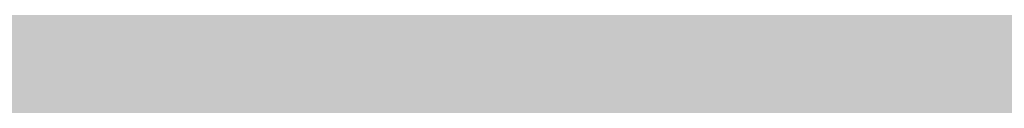
# Model space of a CAD drawing. Units: feet. Extents: x 3168 to 4724, y 827 to 1477.
# Tile 66 of 256: x 3273.15625 to 3273.17306, y 1099.01485 to 1099.01628. Entities that reach past the tile are written whole.
import ezdxf

# ---------------------------------------------------------------- set-up
doc = ezdxf.new("R2010")
doc.units = ezdxf.units.FT
doc.layers.add('A-ELEV', color=7, linetype='Continuous', lineweight=35)
doc.layers.add('A-ELEV-PATT', color=8, linetype='Continuous', lineweight=13)

msp = doc.modelspace()

# ---------------------------------------------------------------- hatches: boundary and pattern name
at = {"layer": 'A-ELEV-PATT'}
h = msp.add_hatch(color=256, dxfattribs=at)
h.dxf.hatch_style = 1
edge = h.paths.add_edge_path()
edge.add_ellipse((3552.905762, 979.220141), major_axis=(36.744924, 0), ratio=0.484848485, start_angle=0, end_angle=360)
edge = h.paths.add_edge_path()
edge.add_ellipse((3559.891637, 929.252282), major_axis=(36.744924, 0), ratio=0.484848485, start_angle=0, end_angle=360)
edge = h.paths.add_edge_path()
edge.add_line((3299.31681, 1198.606081), (3479.916714, 1198.606081))
edge.add_line((3479.916714, 1198.606081), (3479.916714, 1209.86857))
edge.add_spline(control_points=[(3479.916714, 1209.86857), (3464.301157, 1209.86857), (3448.685601, 1209.86857), (3410.949139, 1209.86857), (3388.828234, 1209.86857), (3355.646876, 1209.86857), (3344.586423, 1209.86857), (3327.995745, 1209.86857), (3322.465518, 1209.86857), (3314.170179, 1209.86857), (3311.405066, 1209.86857), (3307.257396, 1209.86857), (3305.874839, 1209.86857), (3303.801005, 1209.86857), (3303.109726, 1209.86857), (3302.072809, 1209.86857), (3301.72717, 1209.86857), (3301.208711, 1209.86857), (3301.035891, 1209.86857), (3300.776662, 1209.86857), (3300.690252, 1209.86857), (3300.560638, 1209.86857), (3300.517433, 1209.86857), (3300.452625, 1209.86857), (3300.431023, 1209.86857), (3300.398619, 1209.86857), (3300.387818, 1209.86857), (3300.366216, 1209.86857), (3300.345676, 1209.86857), (3300.345548, 1209.86857), (3300.345505, 1209.86857), (3300.343304, 1209.86857), (3300.341146, 1209.868571), (3300.337909, 1209.868571), (3300.33683, 1209.868572), (3300.333942, 1209.868573), (3300.332133, 1209.868574), (3300.325515, 1209.868577), (3300.320706, 1209.868581), (3300.310925, 1209.868592), (3300.305952, 1209.868598), (3300.290511, 1209.868623), (3300.280045, 1209.868646), (3300.232425, 1209.868777), (3300.195298, 1209.868954), (3299.951068, 1209.870608), (3299.744824, 1209.874326), (3299.436827, 1209.883257), (3299.334389, 1209.886792), (3299.181079, 1209.89292), (3299.130033, 1209.895099), (3298.652217, 1209.916801), (3298.22946, 1209.945718), (3297.601631, 1210.002367), (3297.393404, 1210.023464), (3297.082652, 1210.058309), (3296.979332, 1210.070458), (3296.292954, 1210.154861), (3295.718148, 1210.243356), (3294.868717, 1210.39885), (3294.5877, 1210.454478), (3294.169341, 1210.543349), (3294.030415, 1210.573878), (3291.707149, 1211.1012), (3289.65359, 1211.813435), (3285.776259, 1213.563988), (3283.95141, 1214.603478), (3280.512159, 1216.98008), (3278.897241, 1218.317592), (3276.379914, 1220.829489), (3275.416042, 1221.917738), (3274.039342, 1223.7077), (3273.581043, 1224.349535), (3273.143228, 1225.016316)], knot_values=[39.119033, 39.119033, 39.119033, 39.119033, 39.286353, 39.286353, 39.523379, 39.523379, 39.641892, 39.641892, 39.701148, 39.701148, 39.730777, 39.730777, 39.745591, 39.745591, 39.752998, 39.752998, 39.756701, 39.756701, 39.758553, 39.758553, 39.759479, 39.759479, 39.759942, 39.759942, 39.760173, 39.760173, 39.760289, 39.760289, 39.760405, 39.760405, 39.760463, 39.760463, 39.763389, 39.763389, 39.764851, 39.764851, 39.767304, 39.767304, 39.773825, 39.773825, 39.78057, 39.78057, 39.79477, 39.79477, 39.845194, 39.845194, 40.126715, 40.126715, 40.267476, 40.267476, 40.337856, 40.337856, 40.927023, 40.927023, 41.221606, 41.221606, 41.368898, 41.368898, 42.202622, 42.202622, 42.619485, 42.619485, 42.827916, 42.827916, 46.118323, 46.118323, 49.408731, 49.408731, 52.699139, 52.699139, 54.927489, 54.927489, 56.104228, 56.104228, 56.104228, 56.104228], weights=[1, 1, 1, 1, 1, 1, 1, 1, 1, 1, 1, 1, 1, 1, 1, 1, 1, 1, 1, 1, 1, 1, 1, 1, 1, 1, 1, 1, 1, 1, 1, 1, 1, 1, 1, 1, 1, 1, 1, 1, 1, 1, 1, 1, 1, 1, 1, 1, 1, 1, 1, 1, 1, 1, 1, 1, 1, 1, 1, 1, 1, 1, 1, 1, 1, 1, 1, 1, 1, 1, 1, 1, 1, 1], degree=3, periodic=0)
edge.add_line((3273.143228, 1225.016316), (3273.143228, 1099.016316))
edge.add_line((3273.143228, 1099.016316), (3299.31681, 1099.016316))
edge.add_line((3299.31681, 1099.016316), (3299.31681, 1198.606081))
edge = h.paths.add_edge_path()
edge.add_line((3304.758443, 1324.15806), (3479.916714, 1324.15806))
edge.add_line((3479.916714, 1324.15806), (3479.916714, 1335.714618))
edge.add_line((3479.916714, 1335.714618), (3269.161628, 1335.714618))
edge.add_spline(control_points=[(3269.161628, 1335.714618), (3264.024231, 1335.714618), (3258.364118, 1328.958189), (3259.264311, 1323.900274)], knot_values=[0, 0, 0, 0, 15.412191, 15.412191, 15.412191, 15.412191], degree=3, periodic=0)
edge.add_line((3259.264311, 1323.900274), (3265.516849, 1288.769135))
edge.add_line((3265.516849, 1288.769135), (3275.265103, 1261.545626))
edge.add_line((3275.265103, 1261.545626), (3304.758443, 1261.545626))
edge.add_line((3304.758443, 1261.545626), (3304.758443, 1324.15806))
h = msp.add_hatch(color=256, dxfattribs=at)
h.dxf.hatch_style = 1
h.paths.add_polyline_path([(3384.525247, 1099.016316), (3335.029168, 1099.016316), (3299.31681, 1099.016316), (3273.143228, 1099.016316), (3217.565364, 1099.016316), (3168.069285, 827.11626), (3335.029168, 827.11626)])

# ---------------------------------------------------------------- linework, layer by layer
at = {"layer": 'A-ELEV'}
msp.add_open_spline([(3808.5202, 1099.016316), (3808.5202, 1141.413235), (3808.5202, 1183.810154), (3808.5202, 1226.635324), (3808.5202, 1227.063576), (3808.5202, 1227.491828), (3811.491871, 1248.994673), (3814.463542, 1270.497518), (3817.46523, 1292.217564), (3817.495247, 1292.434764), (3817.525264, 1292.651964), (3817.572801, 1310.106748), (3817.620339, 1327.561532), (3817.667877, 1345.016316), (3817.667877, 1345.457962), (3817.667877, 1345.899608), (3817.667877, 1346.456047), (3817.667877, 1346.57084), (3817.667877, 1346.752887), (3817.667877, 1346.820142), (3817.667877, 1346.93487), (3817.667877, 1346.982345), (3817.667877, 1347.038587), (3817.667877, 1347.047356), (3817.667877, 1347.073661), (3817.667877, 1347.059303), (3817.667877, 1347.061545), (3817.667876, 1347.062667), (3817.667875, 1347.066031), (3817.667874, 1347.068274), (3817.66787, 1347.075001), (3817.667866, 1347.079486), (3817.667849, 1347.092937), (3817.667833, 1347.101902), (3817.667766, 1347.12879), (3817.667699, 1347.146705), (3817.667432, 1347.200421), (3817.667165, 1347.236192), (3817.6661, 1347.343385), (3817.665038, 1347.414686), (3817.660812, 1347.628095), (3817.656608, 1347.769708), (3817.63997, 1348.192487), (3817.623509, 1348.471586), (3817.559094, 1349.300067), (3817.496121, 1349.840588), (3817.255432, 1351.424156), (3817.026318, 1352.428785), (3816.306871, 1354.888914), (3815.743745, 1356.268727), (3814.463959, 1358.81921), (3813.746413, 1359.990968), (3812.195838, 1362.172343), (3811.362245, 1363.182124), (3809.588836, 1365.069009), (3808.648816, 1365.946105), (3806.654262, 1367.579616), (3805.599702, 1368.336154), (3803.352891, 1369.722327), (3802.160535, 1370.352386), (3799.600813, 1371.453586), (3798.232688, 1371.925481), (3795.280084, 1372.634624), (3793.693148, 1372.872068), (3791.869441, 1372.92648), (3791.740861, 1372.92922), (3791.353371, 1372.934101), (3791.092707, 1372.932901), (3790.304116, 1372.915068), (3789.769543, 1372.884195), (3789.20919, 1372.830236), (3789.190622, 1372.828424), (3789.134892, 1372.822912), (3789.097705, 1372.819137), (3789.048445, 1372.814008), (3789.0364, 1372.812743), (3789.000256, 1372.808918), (3788.976147, 1372.806325), (3788.949405, 1372.803404), (3788.946786, 1372.803118), (3788.942567, 1372.802655), (3788.940967, 1372.80248), (3788.938572, 1372.802217), (3788.937777, 1372.802129), (3788.935391, 1372.801867), (3788.867535, 1372.794402), (3788.756866, 1372.782228), (3788.701532, 1372.776141), (3788.53553, 1372.75788), (3788.424861, 1372.745707), (3788.092856, 1372.709185), (3787.871519, 1372.684837), (3787.207509, 1372.611793), (3786.764835, 1372.563097), (3785.436814, 1372.417009), (3784.551467, 1372.319617), (3781.895425, 1372.027442), (3780.12473, 1371.832658), (3774.812646, 1371.248307), (3771.271256, 1370.858739), (3760.647088, 1369.690037), (3753.56431, 1368.910902), (3732.315973, 1366.573498), (3718.150416, 1365.015228), (3694.006758, 1362.359326), (3684.028657, 1361.261694), (3674.050557, 1360.164062), (3664.600662, 1360.164062), (3655.150767, 1360.164062), (3626.801081, 1360.164062), (3607.901291, 1360.164062), (3551.20192, 1360.164062), (3513.40234, 1360.164062), (3467.725182, 1360.164062), (3459.847604, 1360.164062), (3436.214873, 1360.164062), (3420.459718, 1360.164062), (3373.194255, 1360.164062), (3341.683946, 1360.164062), (3302.848162, 1360.164062), (3295.522686, 1360.164062), (3286.038292, 1360.164062), (3283.879372, 1360.164062), (3277.402613, 1360.164062), (3273.084773, 1360.164062), (3267.732851, 1360.164062), (3266.698768, 1360.164062), (3263.59652, 1360.164062), (3261.528355, 1360.164062), (3259.236943, 1360.164062), (3259.013697, 1360.164062), (3258.343958, 1360.164062), (3257.897466, 1360.164062), (3257.430998, 1360.164062), (3257.411022, 1360.164062), (3257.370573, 1360.164062), (3257.37547, 1360.164062), (3257.374598, 1360.164062), (3257.373937, 1360.164062), (3257.371956, 1360.164062), (3257.370635, 1360.164061), (3257.366673, 1360.16406), (3257.364032, 1360.164059), (3257.356109, 1360.164053), (3257.350828, 1360.164047), (3257.334987, 1360.164023), (3257.32443, 1360.163998), (3257.292769, 1360.163899), (3257.271676, 1360.163799), (3257.208439, 1360.163398), (3257.166337, 1360.162995), (3257.040206, 1360.161388), (3256.956349, 1360.159783), (3256.705504, 1360.153393), (3256.53924, 1360.147036), (3256.04357, 1360.121916), (3255.717296, 1360.097102), (3254.752446, 1360.000481), (3254.127968, 1359.906513), (3252.180067, 1359.525332), (3250.941574, 1359.143991), (3248.670175, 1358.24329), (3247.635739, 1357.723834), (3245.732632, 1356.603471), (3244.863388, 1356.00206), (3243.253108, 1354.742865), (3242.511972, 1354.084731), (3240.751052, 1352.344781), (3239.800961, 1351.229574), (3238.087769, 1348.87244), (3237.324685, 1347.630355), (3235.98251, 1344.971632), (3235.402205, 1343.554907), (3234.591081, 1340.815458), (3234.310882, 1339.54355), (3233.97649, 1336.802561), (3233.922113, 1335.330877), (3234.148916, 1332.591269), (3234.349529, 1331.367201), (3234.719893, 1329.999367), (3234.752423, 1329.883362), (3234.853619, 1329.534797), (3234.925892, 1329.301685), (3235.024836, 1329.002552), (3235.046924, 1328.936928), (3235.077639, 1328.847239), (3235.085924, 1328.823198), (3235.110939, 1328.751064), (3235.127828, 1328.702962), (3235.147992, 1328.646242), (3235.151059, 1328.637632), (3235.156096, 1328.623526), (3235.158061, 1328.61803), (3235.160209, 1328.61203), (3235.165612, 1328.596943), (3235.180099, 1328.556486), (3235.190263, 1328.528101), (3235.220756, 1328.442946), (3235.241084, 1328.386176), (3235.302069, 1328.215865), (3235.342726, 1328.102325), (3235.464696, 1327.761704), (3235.54601, 1327.534623), (3235.78995, 1326.853381), (3235.952577, 1326.39922), (3236.440459, 1325.036736), (3236.765713, 1324.128414), (3237.741475, 1321.403446), (3238.391983, 1319.586801), (3240.343508, 1314.136866), (3241.644525, 1310.503576), (3245.547574, 1299.603706), (3248.149607, 1292.337126), (3255.955706, 1270.537385), (3261.159772, 1256.004225), (3267.387618, 1238.612001), (3268.411397, 1235.752937), (3269.510378, 1232.683864), (3269.585579, 1232.473854), (3269.706612, 1232.135851), (3269.752444, 1232.007857), (3269.827329, 1231.79873), (3269.856382, 1231.717595), (3269.906325, 1231.578122), (3269.927215, 1231.519782), (3269.972468, 1231.393406), (3269.996831, 1231.325368), (3270.026503, 1231.242506), (3270.031811, 1231.227681), (3270.040282, 1231.204024), (3270.039224, 1231.206979), (3270.039359, 1231.206601), (3270.039427, 1231.206412), (3270.03963, 1231.205846), (3270.039765, 1231.205468), (3270.040171, 1231.204335), (3270.040442, 1231.203579), (3270.041254, 1231.201313), (3270.041796, 1231.199802), (3270.04342, 1231.195269), (3270.044504, 1231.192248), (3270.047756, 1231.183185), (3270.049926, 1231.177145), (3270.056442, 1231.159028), (3270.060793, 1231.146957), (3270.073867, 1231.110761), (3270.082613, 1231.086656), (3270.108936, 1231.014413), (3270.1266, 1230.96635), (3270.179934, 1230.822457), (3270.215947, 1230.726923), (3270.325323, 1230.441508), (3270.400026, 1230.252811), (3270.629249, 1229.691444), (3270.788883, 1229.323501), (3271.286488, 1228.238319), (3271.6431, 1227.539755), (3272.775859, 1225.515277), (3273.614169, 1224.260502), (3275.416042, 1221.917738), (3276.379914, 1220.829489), (3278.897241, 1218.317592), (3280.512159, 1216.98008), (3283.95141, 1214.603478), (3285.776259, 1213.563988), (3289.65359, 1211.813435), (3291.707149, 1211.1012), (3294.030415, 1210.573878), (3294.169341, 1210.543349), (3294.5877, 1210.454478), (3294.868717, 1210.39885), (3295.718148, 1210.243356), (3296.292954, 1210.154861), (3296.979332, 1210.070458), (3297.082652, 1210.058309), (3297.393404, 1210.023464), (3297.601631, 1210.002367), (3298.22946, 1209.945718), (3298.652217, 1209.916801), (3299.130033, 1209.895099), (3299.181079, 1209.89292), (3299.334389, 1209.886792), (3299.436827, 1209.883257), (3299.744824, 1209.874326), (3299.951068, 1209.870608), (3300.195298, 1209.868954), (3300.232425, 1209.868777), (3300.280045, 1209.868646), (3300.290511, 1209.868623), (3300.305952, 1209.868598), (3300.310925, 1209.868592), (3300.320706, 1209.868581), (3300.325515, 1209.868577), (3300.332133, 1209.868574), (3300.333942, 1209.868573), (3300.33683, 1209.868572), (3300.337909, 1209.868571), (3300.341146, 1209.868571), (3300.343304, 1209.86857), (3300.345505, 1209.86857), (3300.345548, 1209.86857), (3300.345676, 1209.86857), (3300.366216, 1209.86857), (3300.387818, 1209.86857), (3300.398619, 1209.86857), (3300.431023, 1209.86857), (3300.452625, 1209.86857), (3300.517433, 1209.86857), (3300.560638, 1209.86857), (3300.690252, 1209.86857), (3300.776662, 1209.86857), (3301.035891, 1209.86857), (3301.208711, 1209.86857), (3301.72717, 1209.86857), (3302.072809, 1209.86857), (3303.109726, 1209.86857), (3303.801005, 1209.86857), (3305.874839, 1209.86857), (3307.257396, 1209.86857), (3311.405066, 1209.86857), (3314.170179, 1209.86857), (3322.465518, 1209.86857), (3327.995745, 1209.86857), (3344.586423, 1209.86857), (3355.646876, 1209.86857), (3388.828234, 1209.86857), (3410.949139, 1209.86857), (3477.311855, 1209.86857), (3521.553665, 1209.86857), (3566.836184, 1209.86857), (3567.876892, 1209.86857), (3570.999017, 1209.86857), (3573.080433, 1209.86857), (3575.781396, 1209.86857), (3576.400943, 1209.86857), (3577.295821, 1209.86857), (3577.571152, 1209.86857), (3578.397146, 1209.86857), (3578.947808, 1209.86857), (3579.756491, 1209.86857), (3580.014511, 1209.86857), (3580.342737, 1209.86857), (3580.326865, 1209.86857), (3580.32717, 1209.86857), (3580.327323, 1209.86857), (3580.327781, 1209.86857), (3580.328086, 1209.86857), (3580.329002, 1209.86857), (3580.329613, 1209.86857), (3580.331445, 1209.86857), (3580.332667, 1209.86857), (3580.336332, 1209.868569), (3580.338775, 1209.868567), (3580.346107, 1209.868563), (3580.350995, 1209.868558), (3580.365663, 1209.86854), (3580.375445, 1209.868522), (3580.404801, 1209.868449), (3580.424386, 1209.868376), (3580.483183, 1209.868085), (3580.522437, 1209.867793), (3580.640361, 1209.866624), (3580.719195, 1209.865454), (3580.956315, 1209.860766), (3581.115222, 1209.85607), (3581.594164, 1209.83723), (3581.916419, 1209.818331), (3582.889947, 1209.742428), (3583.547986, 1209.666169), (3585.531827, 1209.360617), (3586.867216, 1209.053886), (3589.471545, 1208.252472), (3590.740241, 1207.757852), (3591.995451, 1207.158802), (3592.057809, 1207.12874), (3592.244242, 1207.037954), (3592.367676, 1206.976632), (3592.73528, 1206.790359), (3592.976752, 1206.663101), (3593.244539, 1206.516441), (3593.274731, 1206.499825), (3593.365115, 1206.449839), (3593.425113, 1206.416333), (3593.604314, 1206.315285), (3593.722725, 1206.247211), (3593.857212, 1206.168398), (3593.874362, 1206.158319), (3593.925741, 1206.128041), (3593.959899, 1206.107798), (3594.062086, 1206.046899), (3594.129827, 1206.006074), (3594.208436, 1205.958171), (3594.219683, 1205.951304), (3594.253391, 1205.930686), (3594.275819, 1205.916917), (3594.342972, 1205.875536), (3594.387563, 1205.847853), (3594.433616, 1205.81905), (3594.435256, 1205.818024), (3594.440175, 1205.814946), (3594.443453, 1205.812894), (3594.447123, 1205.810594), (3594.447516, 1205.810348), (3594.448695, 1205.80961), (3594.449481, 1205.809117), (3594.450366, 1205.808562), (3594.450466, 1205.8085), (3594.4506, 1205.808415), (3594.467399, 1205.797887), (3594.493269, 1205.781674), (3594.506204, 1205.773568), (3594.545008, 1205.749248), (3594.570878, 1205.733035), (3594.648487, 1205.684396), (3594.700226, 1205.651969), (3594.855444, 1205.554691), (3594.958922, 1205.489839), (3595.269357, 1205.295282), (3595.476314, 1205.165577), (3596.097185, 1204.776463), (3596.511099, 1204.517054), (3597.752841, 1203.738826), (3598.580669, 1203.220007), (3601.064152, 1201.663551), (3602.719807, 1200.625914), (3607.686774, 1197.513002), (3610.998085, 1195.437727), (3620.932018, 1189.211903), (3627.55464, 1185.061354), (3647.422507, 1172.609707), (3660.667751, 1164.308608), (3700.403484, 1139.405313), (3726.893973, 1122.803116), (3757.205715, 1103.806052), (3761.02697, 1101.411184), (3764.848224, 1099.016316), (3745.328271, 1099.016316), (3725.808319, 1099.016316), (3706.288366, 1099.016316), (3706.288366, 1108.453237), (3706.288366, 1117.890158), (3706.288366, 1127.327079), (3710.750754, 1127.327079), (3715.213143, 1127.327079), (3719.675531, 1127.327079)], degree=3, knots=[0, 0, 0, 0, 0.982037, 0.982037, 0.991957, 0.991957, 0.991957, 1.966522, 1.966522, 1.976367, 1.976367, 1.976367, 2.976367, 2.976367, 2.976367, 3.00169, 3.00169, 3.008272, 3.008272, 3.012129, 3.012129, 3.014851, 3.014851, 3.015353, 3.015353, 3.016359, 3.016359, 3.017365, 3.017365, 3.019376, 3.019376, 3.023398, 3.023398, 3.031442, 3.031442, 3.047531, 3.047531, 3.079708, 3.079708, 3.144063, 3.144063, 3.272772, 3.272772, 3.53019, 3.53019, 4.045026, 4.045026, 5.074698, 5.074698, 6.700878, 6.700878, 8.327058, 8.327058, 9.953238, 9.953238, 11.579418, 11.579418, 13.205598, 13.205598, 14.831778, 14.831778, 16.457958, 16.457958, 18.084138, 18.084138, 18.206872, 18.206872, 18.45234, 18.45234, 18.943275, 18.943275, 18.960093, 18.960093, 18.993729, 18.993729, 19.00461, 19.00461, 19.026374, 19.026374, 19.028737, 19.028737, 19.03018, 19.03018, 19.030897, 19.030897, 19.032332, 19.032332, 19.033766, 19.033766, 19.036636, 19.036636, 19.042374, 19.042374, 19.053851, 19.053851, 19.076805, 19.076805, 19.122714, 19.122714, 19.21453, 19.21453, 19.398163, 19.398163, 19.765429, 19.765429, 20.024128, 20.024128, 20.024128, 20.092031, 20.092031, 20.227836, 20.227836, 20.499446, 20.499446, 20.556051, 20.556051, 20.66926, 20.66926, 20.895678, 20.895678, 20.948316, 20.948316, 20.963829, 20.963829, 20.994855, 20.994855, 21.002285, 21.002285, 21.017146, 21.017146, 21.01875, 21.01875, 21.021959, 21.021959, 21.022102, 21.022102, 21.022249, 21.022249, 21.022708, 21.022708, 21.023627, 21.023627, 21.025464, 21.025464, 21.029138, 21.029138, 21.036486, 21.036486, 21.051183, 21.051183, 21.080575, 21.080575, 21.139361, 21.139361, 21.256932, 21.256932, 21.492073, 21.492073, 21.962356, 21.962356, 23.01002, 23.01002, 24.057684, 24.057684, 25.105348, 25.105348, 26.153011, 26.153011, 27.776787, 27.776787, 29.400562, 29.400562, 31.024337, 31.024337, 32.278801, 32.278801, 33.533265, 33.533265, 34.467568, 34.467568, 34.553971, 34.553971, 34.726776, 34.726776, 34.775309, 34.775309, 34.793079, 34.793079, 34.82862, 34.82862, 34.834979, 34.834979, 34.839039, 34.839039, 34.839411, 34.839411, 34.840285, 34.840285, 34.842034, 34.842034, 34.845531, 34.845531, 34.852525, 34.852525, 34.866512, 34.866512, 34.894488, 34.894488, 34.950439, 34.950439, 35.062342, 35.062342, 35.286147, 35.286147, 35.733758, 35.733758, 35.821815, 35.821815, 35.828283, 35.828283, 35.832225, 35.832225, 35.834724, 35.834724, 35.836521, 35.836521, 35.838617, 35.838617, 35.839073, 35.839073, 35.839345, 35.839345, 35.839617, 35.839617, 35.840161, 35.840161, 35.841249, 35.841249, 35.843425, 35.843425, 35.847778, 35.847778, 35.856482, 35.856482, 35.873891, 35.873891, 35.908709, 35.908709, 35.978345, 35.978345, 36.117617, 36.117617, 36.396161, 36.396161, 36.953248, 36.953248, 38.067423, 38.067423, 40.295772, 40.295772, 42.524122, 42.524122, 45.81453, 45.81453, 49.104937, 49.104937, 52.395345, 52.395345, 52.603776, 52.603776, 53.020639, 53.020639, 53.854363, 53.854363, 54.001655, 54.001655, 54.296238, 54.296238, 54.885405, 54.885405, 54.955785, 54.955785, 55.096546, 55.096546, 55.378067, 55.378067, 55.42849, 55.42849, 55.442691, 55.442691, 55.449436, 55.449436, 55.455957, 55.455957, 55.458409, 55.458409, 55.459872, 55.459872, 55.462798, 55.462798, 55.462856, 55.462856, 55.462972, 55.462972, 55.463088, 55.463088, 55.463319, 55.463319, 55.463782, 55.463782, 55.464708, 55.464708, 55.46656, 55.46656, 55.470263, 55.470263, 55.47767, 55.47767, 55.492484, 55.492484, 55.522112, 55.522112, 55.581369, 55.581369, 55.699882, 55.699882, 55.936907, 55.936907, 56.410959, 56.410959, 56.42211, 56.42211, 56.444413, 56.444413, 56.451051, 56.451051, 56.454001, 56.454001, 56.459901, 56.459901, 56.462666, 56.462666, 56.463418, 56.463418, 56.464171, 56.464171, 56.465675, 56.465675, 56.468684, 56.468684, 56.474702, 56.474702, 56.486738, 56.486738, 56.51081, 56.51081, 56.558955, 56.558955, 56.655243, 56.655243, 56.847821, 56.847821, 57.232975, 57.232975, 58.003284, 58.003284, 59.543901, 59.543901, 62.625137, 62.625137, 68.787607, 68.787607, 74.950078, 74.950078, 75.27336, 75.27336, 75.919923, 75.919923, 77.213051, 77.213051, 77.377769, 77.377769, 77.707206, 77.707206, 78.366079, 78.366079, 78.462532, 78.462532, 78.655436, 78.655436, 79.041245, 79.041245, 79.105735, 79.105735, 79.234714, 79.234714, 79.492672, 79.492672, 79.502197, 79.502197, 79.521249, 79.521249, 79.523534, 79.523534, 79.528103, 79.528103, 79.528682, 79.528682, 79.528885, 79.528885, 79.529089, 79.529089, 79.529495, 79.529495, 79.530308, 79.530308, 79.531935, 79.531935, 79.535187, 79.535187, 79.541693, 79.541693, 79.554704, 79.554704, 79.580725, 79.580725, 79.632769, 79.632769, 79.736856, 79.736856, 79.94503, 79.94503, 80.361377, 80.361377, 80.421435, 80.421435, 80.421435, 81.421435, 81.421435, 81.421435, 82.421435, 82.421435, 82.421435, 83.421435, 83.421435, 83.421435, 83.421435], dxfattribs=at)

doc.saveas('drawing.dxf')
